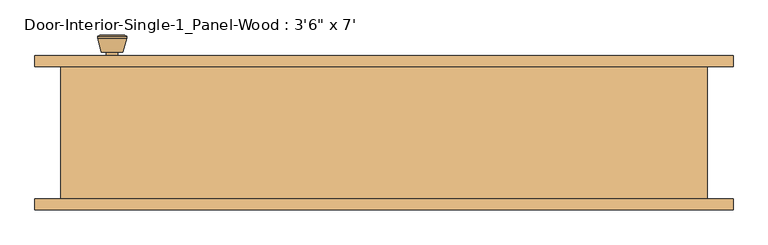
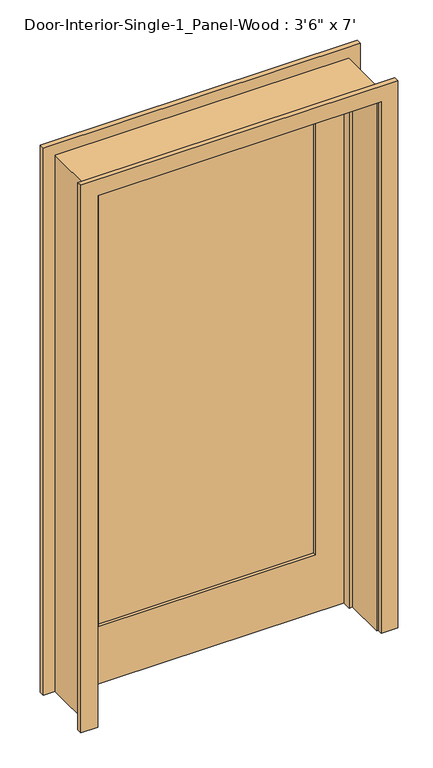
"""IFC4 building model written with IfcOpenShell, lengths in millimetres: door geometry."""

from ifc_helpers import new_model, si_unit, point, frame, frame_2d, origin, place, context, project, spatial, polyline, circle_curve, trimmed, segment, composite_curve, outline, extrude, faceted_brep, source, transform, mapped, element, save
from ifc_brep_helpers import plane_surface, cylinder_surface, revolved_surface, advanced_brep


def door_103cf79b(model_context):
    return source(origin(), model_context, "Body", "SolidModel", [
        advanced_brep(
        [(-469.9, 70.2, 914.4), (-459.9, 70.2, 914.4), (-479.9, 70.2, 914.4), (-449.4241324, 21.2, 914.4), (-469.9, 21.2, 914.4), (-490.3758676, 21.2, 914.4), (-444.9, 23.0278681, 914.4), (-494.9, 23.0278681, 914.4), (-444.9, 26.4915463, 914.4), (-494.9, 26.4915463, 914.4), (-451.263764, 51.2, 914.4), (-488.536236, 51.2, 914.4), (-459.9, 51.2, 914.4), (-479.9, 51.2, 914.4)],
        [
            (0, 1),
            (1, 2, circle_curve(frame((-469.9, 70.2, 914.4), z_axis=(0.0, 1.0, 0.0), x_axis=(-1.0, 0.0, 0.0)), 10.0)),
            (2, 0),
            (2, 1, circle_curve(frame((-469.9, 70.2, 914.4), z_axis=(0.0, 1.0, 0.0), x_axis=(-1.0, 0.0, 0.0)), 10.0)),
            (3, 4),
            (4, 5),
            (5, 3, circle_curve(frame((-469.9, 21.2, 914.4), z_axis=(0.0, -1.0, 0.0), x_axis=(-1.0, 0.0, 0.0)), 20.4758676)),
            (3, 5, circle_curve(frame((-469.9, 21.2, 914.4), z_axis=(0.0, -1.0, 0.0), x_axis=(-1.0, 0.0, 0.0)), 20.4758676)),
            (6, 3),
            (5, 7),
            (7, 6, circle_curve(frame((-469.9, 23.0278681, 914.4), z_axis=(0.0, -1.0, 0.0), x_axis=(-1.0, 0.0, 0.0)), 25.0)),
            (6, 7, circle_curve(frame((-469.9, 23.0278681, 914.4), z_axis=(0.0, -1.0, 0.0), x_axis=(-1.0, 0.0, 0.0)), 25.0)),
            (8, 6),
            (7, 9),
            (9, 8, circle_curve(frame((-469.9, 26.4915463, 914.4), z_axis=(0.0, -1.0, 0.0), x_axis=(-1.0, 0.0, 0.0)), 25.0)),
            (8, 9, circle_curve(frame((-469.9, 26.4915463, 914.4), z_axis=(0.0, -1.0, 0.0), x_axis=(-1.0, 0.0, 0.0)), 25.0)),
            (10, 8),
            (9, 11),
            (11, 10, circle_curve(frame((-469.9, 51.2, 914.4), z_axis=(0.0, -1.0, 0.0), x_axis=(-1.0, 0.0, 0.0)), 18.636236)),
            (10, 11, circle_curve(frame((-469.9, 51.2, 914.4), z_axis=(0.0, -1.0, 0.0), x_axis=(-1.0, 0.0, 0.0)), 18.636236)),
            (12, 10),
            (11, 13),
            (13, 12, circle_curve(frame((-469.9, 51.2, 914.4), z_axis=(0.0, -1.0, 0.0), x_axis=(-1.0, 0.0, 0.0)), 10.0)),
            (12, 13, circle_curve(frame((-469.9, 51.2, 914.4), z_axis=(0.0, -1.0, 0.0), x_axis=(-1.0, 0.0, 0.0)), 10.0)),
            (1, 12),
            (13, 2),
        ],
        [
            plane_surface(frame((-469.9, 70.2, 914.4), z_axis=(0.0, 1.0, 0.0), x_axis=(-1.0, 0.0, 0.0))),
            plane_surface(frame((-469.9, 21.2, 914.4), z_axis=(0.0, -1.0, 0.0), x_axis=(-1.0, 0.0, 0.0))),
            revolved_surface(polyline([(-490.3758676, 21.2, 914.4), (-494.9, 23.0278681, 914.4)]), (-469.9, 70.2, 914.4), (0.0, 1.0, 0.0)),
            cylinder_surface(frame((-469.9, 70.2, 914.4), z_axis=(0.0, 1.0, 0.0), x_axis=(-1.0, 0.0, 0.0)), 25.0),
            revolved_surface(polyline([(-494.9, 26.4915463, 914.4), (-488.536236, 51.2, 914.4)]), (-469.9, 70.2, 914.4), (0.0, 1.0, 0.0)),
            plane_surface(frame((-469.9, 51.2, 914.4), z_axis=(0.0, 1.0, 0.0), x_axis=(-1.0, 0.0, 0.0))),
            cylinder_surface(frame((-469.9, 70.2, 914.4), z_axis=(0.0, 1.0, 0.0), x_axis=(-1.0, 0.0, 0.0)), 10.0),
        ],
        [
            (0, [[1, 2, 3]]),
            (0, [[-3, 4, -1]]),
            (1, [[5, 6, 7]]),
            (1, [[-6, -5, 8]]),
            (2, [[9, -7, 10, 11]]),
            (2, [[-10, -8, -9, 12]]),
            (3, [[13, -11, 14, 15]]),
            (3, [[-14, -12, -13, 16]]),
            (4, [[17, -15, 18, 19]]),
            (4, [[-18, -16, -17, 20]]),
            (5, [[21, -19, 22, 23]]),
            (5, [[-22, -20, -21, 24]]),
            (6, [[25, -23, 26, -2]]),
            (6, [[-26, -24, -25, -4]]),
        ],
    ),
        extrude(outline(composite_curve([segment(trimmed(circle_curve(frame_2d((914.4, -469.9)), 30.0), [point((914.4, -499.9))], [point((914.4, -439.9))], False, "CARTESIAN"), True, "CONTINUOUS"), segment(trimmed(circle_curve(frame_2d((914.4, -469.9)), 30.0), [point((914.4, -439.9))], [point((914.4, -499.9))], False, "CARTESIAN"), True, "CONTINUOUS")], self_intersect=False)), frame((0.0, 70.2, 0.0), z_axis=(0.0, 1.0, 0.0), x_axis=(0.0, 0.0, 1.0)), (0.0, 0.0, 1.0), 6.0),
        advanced_brep(
        [(-469.9, 117.125, 914.4), (-479.9, 117.125, 914.4), (-459.9, 117.125, 914.4), (-449.4241324, 166.125, 914.4), (-490.3758676, 166.125, 914.4), (-469.9, 166.125, 914.4), (-444.9, 164.2971319, 914.4), (-494.9, 164.2971319, 914.4), (-444.9, 160.8334537, 914.4), (-494.9, 160.8334537, 914.4), (-451.263764, 136.125, 914.4), (-488.536236, 136.125, 914.4), (-459.9, 136.125, 914.4), (-479.9, 136.125, 914.4)],
        [
            (0, 1),
            (1, 2, circle_curve(frame((-469.9, 117.125, 914.4), z_axis=(0.0, -1.0, 0.0), x_axis=(-1.0, 0.0, 0.0)), 10.0)),
            (2, 0),
            (2, 1, circle_curve(frame((-469.9, 117.125, 914.4), z_axis=(0.0, -1.0, 0.0), x_axis=(-1.0, 0.0, 0.0)), 10.0)),
            (3, 4, circle_curve(frame((-469.9, 166.125, 914.4), z_axis=(0.0, 1.0, 0.0), x_axis=(-1.0, 0.0, 0.0)), 20.4758676)),
            (4, 5),
            (5, 3),
            (4, 3, circle_curve(frame((-469.9, 166.125, 914.4), z_axis=(0.0, 1.0, 0.0), x_axis=(-1.0, 0.0, 0.0)), 20.4758676)),
            (6, 7, circle_curve(frame((-469.9, 164.2971319, 914.4), z_axis=(0.0, 1.0, 0.0), x_axis=(-1.0, 0.0, 0.0)), 25.0)),
            (7, 4),
            (3, 6),
            (7, 6, circle_curve(frame((-469.9, 164.2971319, 914.4), z_axis=(0.0, 1.0, 0.0), x_axis=(-1.0, 0.0, 0.0)), 25.0)),
            (8, 9, circle_curve(frame((-469.9, 160.8334537, 914.4), z_axis=(0.0, 1.0, 0.0), x_axis=(-1.0, 0.0, 0.0)), 25.0)),
            (9, 7),
            (6, 8),
            (9, 8, circle_curve(frame((-469.9, 160.8334537, 914.4), z_axis=(0.0, 1.0, 0.0), x_axis=(-1.0, 0.0, 0.0)), 25.0)),
            (10, 11, circle_curve(frame((-469.9, 136.125, 914.4), z_axis=(0.0, 1.0, 0.0), x_axis=(-1.0, 0.0, 0.0)), 18.636236)),
            (11, 9),
            (8, 10),
            (11, 10, circle_curve(frame((-469.9, 136.125, 914.4), z_axis=(0.0, 1.0, 0.0), x_axis=(-1.0, 0.0, 0.0)), 18.636236)),
            (12, 13, circle_curve(frame((-469.9, 136.125, 914.4), z_axis=(0.0, 1.0, 0.0), x_axis=(-1.0, 0.0, 0.0)), 10.0)),
            (13, 11),
            (10, 12),
            (13, 12, circle_curve(frame((-469.9, 136.125, 914.4), z_axis=(0.0, 1.0, 0.0), x_axis=(-1.0, 0.0, 0.0)), 10.0)),
            (1, 13),
            (12, 2),
        ],
        [
            plane_surface(frame((-469.9, 117.125, 914.4), z_axis=(0.0, -1.0, 0.0), x_axis=(-1.0, 0.0, 0.0))),
            plane_surface(frame((-469.9, 166.125, 914.4), z_axis=(0.0, 1.0, 0.0), x_axis=(-1.0, 0.0, 0.0))),
            revolved_surface(polyline([(-490.3758676, 166.125, 914.4), (-494.9, 164.2971319, 914.4)]), (-469.9, 117.125, 914.4), (0.0, -1.0, 0.0)),
            cylinder_surface(frame((-469.9, 117.125, 914.4), z_axis=(0.0, -1.0, 0.0), x_axis=(-1.0, 0.0, 0.0)), 25.0),
            revolved_surface(polyline([(-494.9, 160.8334537, 914.4), (-488.536236, 136.125, 914.4)]), (-469.9, 117.125, 914.4), (0.0, -1.0, 0.0)),
            plane_surface(frame((-469.9, 136.125, 914.4), z_axis=(0.0, -1.0, 0.0), x_axis=(-1.0, 0.0, 0.0))),
            cylinder_surface(frame((-469.9, 117.125, 914.4), z_axis=(0.0, -1.0, 0.0), x_axis=(-1.0, 0.0, 0.0)), 10.0),
        ],
        [
            (0, [[1, 2, 3]]),
            (0, [[-3, 4, -1]]),
            (1, [[5, 6, 7]]),
            (1, [[8, -7, -6]]),
            (2, [[9, 10, -5, 11]]),
            (2, [[12, -11, -8, -10]]),
            (3, [[13, 14, -9, 15]]),
            (3, [[16, -15, -12, -14]]),
            (4, [[17, 18, -13, 19]]),
            (4, [[20, -19, -16, -18]]),
            (5, [[21, 22, -17, 23]]),
            (5, [[24, -23, -20, -22]]),
            (6, [[-2, 25, -21, 26]]),
            (6, [[-4, -26, -24, -25]]),
        ],
    ),
        extrude(outline(composite_curve([segment(trimmed(circle_curve(frame_2d((914.4, -469.9)), 30.0), [point((914.4, -499.9))], [point((914.4, -439.9))], False, "CARTESIAN"), True, "CONTINUOUS"), segment(trimmed(circle_curve(frame_2d((914.4, -469.9)), 30.0), [point((914.4, -439.9))], [point((914.4, -499.9))], False, "CARTESIAN"), True, "CONTINUOUS")], self_intersect=False)), frame((0.0, 111.125, 0.0), z_axis=(0.0, 1.0, 0.0), x_axis=(0.0, 0.0, 1.0)), (0.0, 0.0, 1.0), 6.0),
        faceted_brep([(558.8, 111.125, 0.0), (558.8, -117.475, 0.0), (533.4, -117.475, 0.0), (533.4, 41.275, 0.0), (520.7, 41.275, 0.0), (520.7, 76.2, 0.0), (533.4, 76.2, 0.0), (533.4, 111.125, 0.0), (558.8, 111.125, 2159.0), (558.8, -117.475, 2159.0), (-558.8, -117.475, 2159.0), (-558.8, -117.475, 0.0), (-533.4, -117.475, 0.0), (-533.4, -117.475, 2133.6), (533.4, -117.475, 2133.6), (533.4, 41.275, 2133.6), (-533.4, 41.275, 2133.6), (-533.4, 41.275, 0.0), (-520.7, 41.275, 0.0), (-520.7, 41.275, 2120.9), (520.7, 41.275, 2120.9), (520.7, 76.2, 2120.9), (-520.7, 76.2, 2120.9), (-520.7, 76.2, 0.0), (-533.4, 76.2, 0.0), (-533.4, 76.2, 2133.6), (533.4, 76.2, 2133.6), (533.4, 111.125, 2133.6), (-533.4, 111.125, 2133.6), (-533.4, 111.125, 0.0), (-558.8, 111.125, 0.0), (-558.8, 111.125, 2159.0)], [[[0, 1, 2, 3, 4, 5, 6, 7]], [[1, 0, 8, 9]], [[2, 1, 9, 10, 11, 12, 13, 14]], [[3, 2, 14, 15]], [[4, 3, 15, 16, 17, 18, 19, 20]], [[5, 4, 20, 21]], [[6, 5, 21, 22, 23, 24, 25, 26]], [[7, 6, 26, 27]], [[0, 7, 27, 28, 29, 30, 31, 8]], [[9, 8, 31, 10]], [[15, 14, 13, 16]], [[21, 20, 19, 22]], [[27, 26, 25, 28]], [[30, 29, 24, 23, 18, 17, 12, 11]], [[10, 31, 30, 11]], [[16, 13, 12, 17]], [[22, 19, 18, 23]], [[28, 25, 24, 29]]]),
        extrude(outline(polyline([(2133.6, -533.4), (0.0, -533.4), (0.0, 533.4), (2133.6, 533.4), (2133.6, -533.4)]), holes=[polyline([(2014.5375, -412.75), (2014.5375, 412.75), (231.775, 412.75), (231.775, -412.75), (2014.5375, -412.75)])]), frame((0.0, 76.2, 0.0), z_axis=(0.0, 1.0, 0.0), x_axis=(0.0, 0.0, 1.0)), (0.0, 0.0, 1.0), 34.925),
        extrude(outline(polyline([(412.75, 87.8416667), (-412.75, 87.8416667), (-412.75, 99.4833333), (412.75, 99.4833333), (412.75, 87.8416667)])), frame((0.0, 0.0, 231.775), z_axis=(0.0, 0.0, 1.0), x_axis=(1.0, 0.0, 0.0)), (0.0, 0.0, 1.0), 1782.7625),
        extrude(outline(polyline([(0.0, 539.75), (0.0, 603.25), (2203.45, 603.25), (2203.45, -603.25), (0.0, -603.25), (0.0, -539.75), (2139.95, -539.75), (2139.95, 539.75), (0.0, 539.75)])), frame((0.0, 111.125, 0.0), z_axis=(0.0, 1.0, 0.0), x_axis=(0.0, 0.0, 1.0)), (0.0, 0.0, 1.0), 19.05),
        extrude(outline(polyline([(0.0, 539.75), (0.0, 603.25), (2203.45, 603.25), (2203.45, -603.25), (0.0, -603.25), (0.0, -539.75), (2139.95, -539.75), (2139.95, 539.75), (0.0, 539.75)])), frame((0.0, -136.525, 0.0), z_axis=(0.0, 1.0, 0.0), x_axis=(0.0, 0.0, 1.0)), (0.0, 0.0, 1.0), 19.05),
    ])


if __name__ == "__main__":
    model = new_model("IFC4")
    model_context = context("Model", 3, world=origin())
    ifc_project = project(units=[si_unit("LENGTHUNIT", "METRE", prefix="MILLI")], contexts=[model_context])
    site = spatial("IfcSite", under=ifc_project)
    building = spatial("IfcBuilding", under=site)
    placement = place(None, origin())
    door_shape = door_103cf79b(model_context)
    element("IfcDoor", 1, ObjectType="Door-Interior-Single-1_Panel-Wood : 3'6\" x 7'", at=placement, inside=building, context=model_context, shape_type="MappedRepresentation", body=[
        mapped(door_shape, transform((0.0, 0.0, 0.0), x_axis=(1.0, 0.0, 0.0), y_axis=(0.0, 1.0, 0.0), z_axis=(0.0, 0.0, 1.0))),
    ])
    save(model, "model.ifc")

# Revit data of these elements
# Type "Door-Interior-Single-1_Panel-Wood : 3'6\" x 7'"
#   Type Mark = "9"
#   Assembly Code = "C1020300"
#   Analytic Construction = "Wooden"
#   Top Rail = 0' - 4 11/16"
#   Thickness = 0' - 1 3/8"
#   Thermal Resistance (R) = 2.5876 (h·ft²·°F)/BTU
#   Swing Angle [instance default] = 90.00°
#   Stiles = 0' - 4 3/4"
#   Rough Width = 3' - 8"
#   Rough Height = 7' - 1"
#   Height = 7' - 0"
#   Width = 3' - 6"
#   Heat Transfer Coefficient (U) = 0.3865 BTU/(h·ft²·°F)
#   Bottom Rail = 0' - 9 1/8"
#   Trim Material = Cherry
#   Panel Material = Cherry
#   Frame Material = Cherry
#   Door Handle Material = Aluminum
#   Visual Light Transmittance = 0
#   Solar Heat Gain Coefficient = 0
#   Wall Closure = (empty or 0)
#   Function = (empty or 0)
# Element 1 (IfcDoor, "Door-Interior-Single-1_Panel-Wood : 3'6\" x 7'")
#   Materials on its faces: "Cherry", "Aluminum"
# Materials
#   "Cherry": class "Wood", colour RGB 226 177 128, transparency 0, Description = "Prunus Serotina", Cost = 0
#   "Aluminum": class "Metal", colour RGB 247 247 247, transparency 0, Description = "Aluminum 6061", Cost = 0
